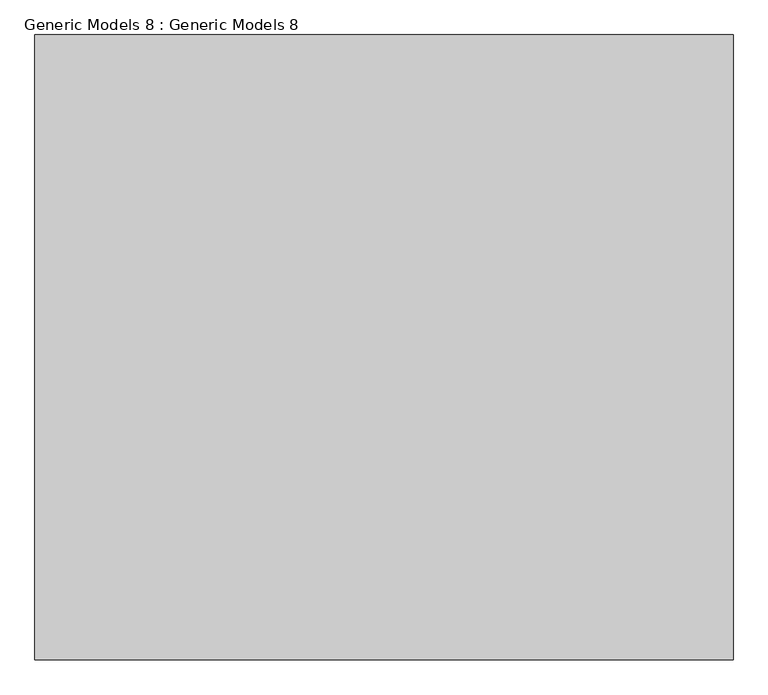
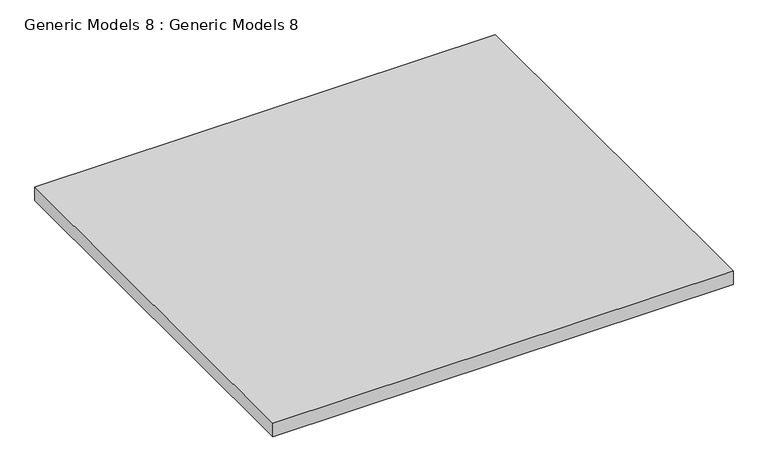
"""IFC4 building model written with IfcOpenShell, lengths in millimetres: proxy geometry, Generic Models 8 : Generic Models 8."""

from ifc_helpers import new_model, si_unit, frame, origin, place, context, project, spatial, polyline, outline, extrude, source, transform, mapped, element, save


def generic_models_8_generic_models_8_5a9fc4db(model_context):
    return source(origin(), model_context, "Body", "SweptSolid", [
        extrude(outline(polyline([(-4797.9586008, -6625.3493461), (-4797.9586008, -2268.3844117), (66.1413992, -2268.3844117), (66.1413992, -6625.3493461), (-4797.9586008, -6625.3493461)])), frame((0.0, 0.0, 6045.2), z_axis=(0.0, 0.0, 1.0), x_axis=(1.0, 0.0, 0.0)), (0.0, 0.0, 1.0), 152.4),
    ])


if __name__ == "__main__":
    model = new_model("IFC4")
    model_context = context("Model", 3, world=origin())
    ifc_project = project(units=[si_unit("LENGTHUNIT", "METRE", prefix="MILLI")], contexts=[model_context])
    site = spatial("IfcSite", under=ifc_project)
    building = spatial("IfcBuilding", under=site)
    placement = place(None, origin())
    generic_models_8_generic_models_8_shape = generic_models_8_generic_models_8_5a9fc4db(model_context)
    element("IfcBuildingElementProxy", 1, Name="Generic Models 8 : Generic Models 8", ObjectType="Generic Models 8 : Generic Models 8", at=placement, inside=building, context=model_context, shape_type="MappedRepresentation", body=[
        mapped(generic_models_8_generic_models_8_shape, transform((0.0, 0.0, 0.0), x_axis=(1.0, 0.0, 0.0), y_axis=(0.0, 1.0, 0.0), z_axis=(0.0, 0.0, 1.0))),
    ])
    save(model, "model.ifc")

# Revit data of these elements
# Element 1 (IfcBuildingElementProxy, "Generic Models 8 : Generic Models 8")
#   Materials on its faces: "wood ceiling"
# Materials
#   "wood ceiling": class "Generic", colour RGB 120 120 120, transparency 0, Cost = 0
